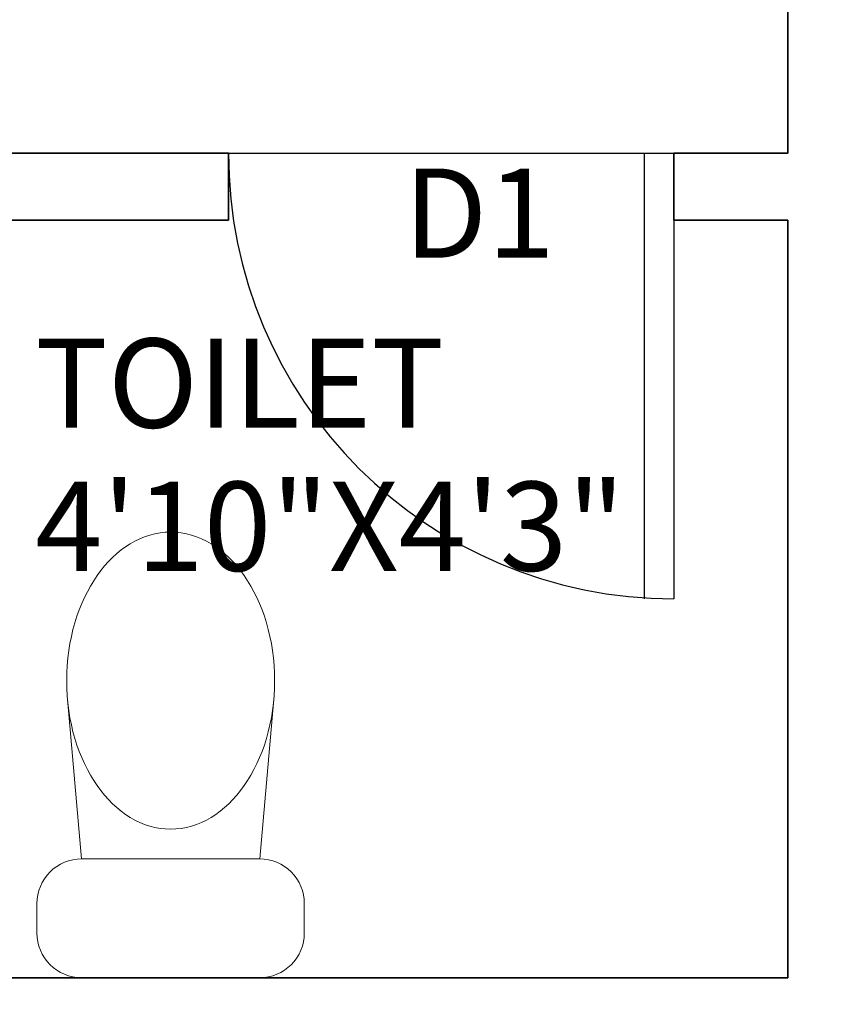
# Model space of a CAD drawing. Units: inches. Extents: x -26 to 575, y -18 to 513.
# Tile 23 of 28: x 385 to 439, y 241 to 307. Entities that reach past the tile are written whole.
import ezdxf

# ---------------------------------------------------------------- set-up
doc = ezdxf.new("R2010")
doc.units = ezdxf.units.IN
doc.header["$MEASUREMENT"] = 0
for name, color, linetype, lineweight in [('A-ANNO-DIMS', 2, 'Continuous', 18), ('A-ANNO-TEXT', 7, 'Continuous', 18), ('A-AREA-IDEN', 7, 'Continuous', 18), ('A-DOOR', 3, 'Continuous', 25), ('A-FLOR-FIXT', 9, 'Continuous', 18), ('A-WALL', 7, 'Continuous', 35)]:
    doc.layers.add(name, color=color, linetype=linetype, lineweight=lineweight)
doc.styles.get("Standard").update_dxf_attribs({"font": 'arial.ttf', "height": 6})
doc.dimstyles.get("Standard").update_dxf_attribs({"dimtxt": 6, "dimasz": 0.18, "dimexe": 0.18, "dimexo": 0.0625, "dimgap": 0.09, "dimtad": 0, "dimtih": 1, "dimtoh": 1, "dimzin": 0, "dimdsep": 46, "dimlunit": 3, "dimtxsty": 'Standard', "dimcen": 0.09, "dimadec": 0, "dimazin": 0, "dimtfac": 1, "dimtofl": 0, "dimtmove": 0, "dimatfit": 3, "dimfxl": 1, "dimtolj": 1, "dimtzin": 0, "dimarcsym": 0})

# ---------------------------------------------------------------- blocks, each defined once
blk = doc.blocks.new('DOOR-SWING-30IN')
for p, q in [((-30, 0), (0, 0)), ((-2, 0), (-2, -30)), ((0, 0), (0, -30))]:
    blk.add_line(p, q)
blk.add_arc((0, 0), 30, 180, 270)
blk = doc.blocks.new('WC-FLOOR-MOUNT')
for p, q in [((-6, 8), (-6.945, 18.754)), ((6, 8), (6.945, 18.754))]:
    blk.add_line(p, q)
blk.add_lwpolyline([(-6, 8), (6, 8, -0.414214), (9, 5), (9, 3, -0.414214), (6, 0), (-6, 0, -0.414214), (-9, 3), (-9, 5, -0.414214)], format="xyb", close=True)
blk.add_ellipse((0, 20), major_axis=(0, 10), ratio=0.7)
blk = doc.blocks.new('*D14')
at = {"layer": 'A-ANNO-DIMS', "color": 0, "lineweight": -2, "transparency": 16777216}
for p, q in [((385.797, 329.945), (385.797, 323.528)), ((427.797, 329.945), (427.797, 323.528)), ((385.977, 323.708), (427.617, 323.708)), ((427.797, 323.708), (427.977, 323.708))]:
    blk.add_line(p, q, dxfattribs=at)
at = {"layer": 'A-ANNO-DIMS', "color": 0, "transparency": 16777216}
for points in [[(385.977, 323.738), (385.977, 323.678), (385.797, 323.708)], [(427.617, 323.738), (427.617, 323.678), (427.797, 323.708)]]:
    blk.add_solid(points, dxfattribs=at)
at = {"layer": 'Defpoints', "color": 0, "transparency": 16777216}
for p in [(385.797, 330.008), (427.797, 330.008), (427.797, 323.708)]:
    blk.add_point(p, dxfattribs=at)
at = {"layer": 'A-ANNO-DIMS', "color": 0, "transparency": 16777216, "insert": (464.132, 323.708), "char_height": 6, "attachment_point": 5}
blk.add_mtext('\\A1;DOOR D 3\'-6" TYP.', dxfattribs=at)
blk = doc.blocks.new('*D26')
at = {"layer": 'A-ANNO-DIMS', "color": 0, "lineweight": -2, "transparency": 16777216}
for p, q in [((337.628, 252.609), (352.461, 252.609)), ((352.281, 252.429), (352.281, 206.753)), ((352.281, 154.689), (352.281, 200.364)), ((337.628, 154.509), (352.461, 154.509))]:
    blk.add_line(p, q, dxfattribs=at)
at = {"layer": 'A-ANNO-DIMS', "color": 0, "transparency": 16777216}
for points in [[(352.251, 252.429), (352.311, 252.429), (352.281, 252.609)], [(352.251, 154.689), (352.311, 154.689), (352.281, 154.509)]]:
    blk.add_solid(points, dxfattribs=at)
at = {"layer": 'Defpoints', "color": 0, "transparency": 16777216}
for p in [(337.566, 252.609), (352.281, 252.609), (337.566, 154.509)]:
    blk.add_point(p, dxfattribs=at)
at = {"layer": 'A-ANNO-DIMS', "color": 0, "transparency": 16777216, "insert": (352.281, 203.559), "char_height": 6, "attachment_point": 5}
blk.add_mtext('\\A1;SECTIONAL SOFA 8\'-2" TYP.', dxfattribs=at)

msp = doc.modelspace()

# ---------------------------------------------------------------- linework, layer by layer
at = {"layer": 'A-WALL'}
for p, q in [((436.677, 298.508), (436.677, 330.008)), ((399.008, 298.508), (374.177, 298.508)), ((399.008, 294.008), (399.008, 298.508)), ((436.677, 298.508), (429.008, 298.508)), ((429.008, 294.008), (429.008, 298.508)), ((399.008, 294.008), (378.677, 294.008)), ((436.677, 294.008), (429.008, 294.008)), ((436.677, 243.008), (436.677, 294.008)), ((436.677, 243.008), (378.677, 243.008))]:
    msp.add_line(p, q, dxfattribs=at)

# ---------------------------------------------------------------- block references
at = {"layer": 'A-DOOR'}
msp.add_blockref('DOOR-SWING-30IN', (429.008, 298.508), dxfattribs=at)
at = {"layer": 'A-FLOR-FIXT'}
msp.add_blockref('WC-FLOOR-MOUNT', (395.117, 243.008), dxfattribs=at)

# ---------------------------------------------------------------- texts
at = {"layer": 'A-ANNO-TEXT'}
msp.add_text('D1', height=6, rotation=0.00167, dxfattribs=at).set_placement((410.812, 291.475))
at = {"layer": 'A-AREA-IDEN'}
for s, p in [('TOILET', (385.989, 280.033)), ('4\'10"X4\'3"', (385.989, 270.395))]:
    msp.add_text(s, height=6, rotation=0.00167, dxfattribs=at).set_placement(p)

# ---------------------------------------------------------------- dimensions: what is measured, and where the dimension line sits
at = {"layer": 'A-ANNO-DIMS'}
dim = msp.add_linear_dim(base=(427.797, 323.708), p1=(385.797, 330.008), p2=(427.797, 330.008), text='DOOR D <> TYP.', dimstyle='Standard', override={"dimdec": 1, "dimlfac": 1, "dimrnd": 0, "dimzin": 1, "dimdsep": 46, "dimlunit": 4, "dimfrac": 2}, dxfattribs=at)
dim.commit()
dim.dimension.update_dxf_attribs({"geometry": '*D14', "text_midpoint": (464.132, 323.708)})
dim = msp.add_linear_dim(base=(352.281, 252.609), p1=(337.566, 154.509), p2=(337.566, 252.609), angle=90, text='SECTIONAL SOFA <> TYP.', dimstyle='Standard', override={"dimdec": 1, "dimlfac": 1, "dimrnd": 0, "dimzin": 1, "dimdsep": 46, "dimlunit": 4, "dimfrac": 2}, dxfattribs=at)
dim.commit()
dim.dimension.update_dxf_attribs({"geometry": '*D26', "text_midpoint": (352.281, 203.559)})

doc.saveas('drawing.dxf')
